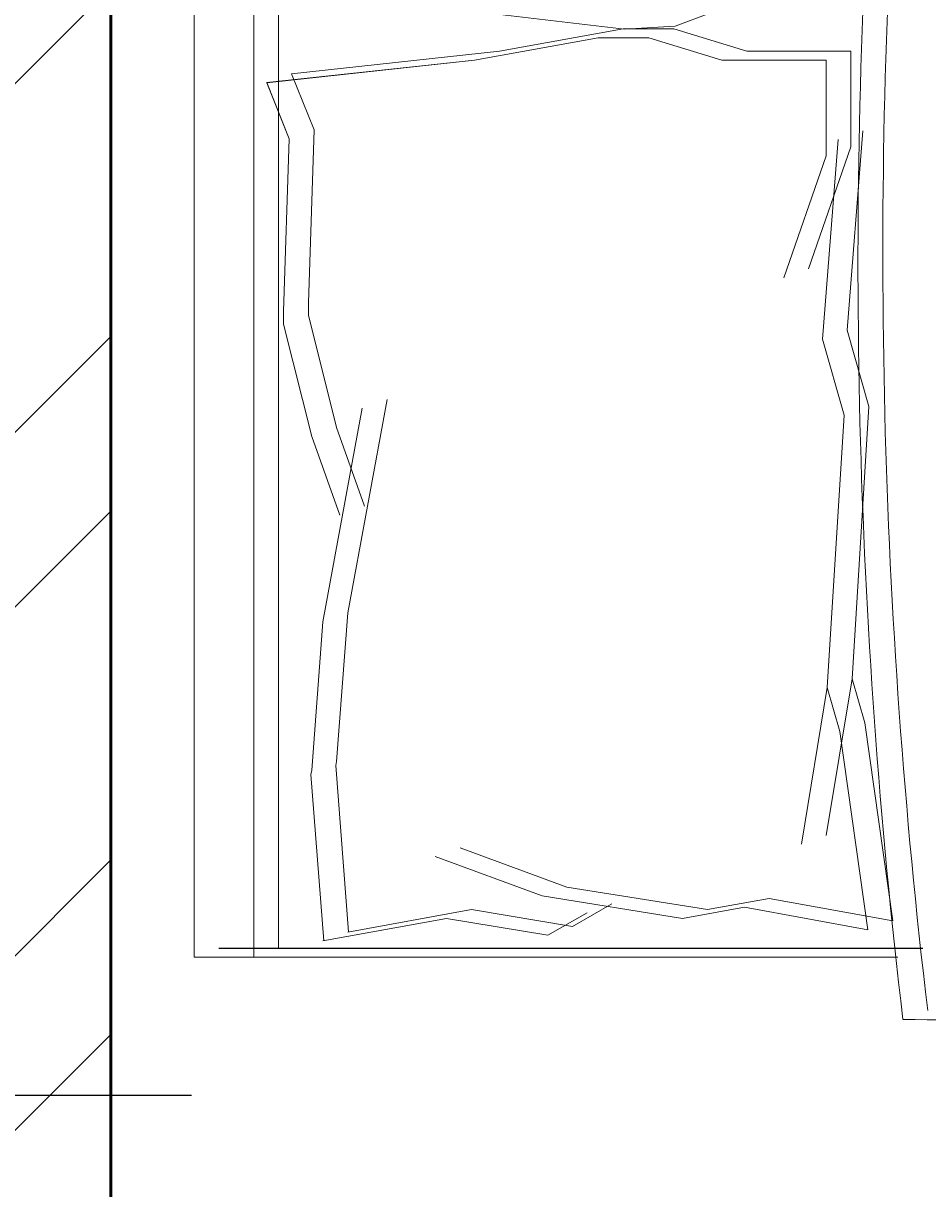
# Model space of a CAD drawing. Units: inches. Extents: x 963 to 2075, y 289 to 2657.
# Tile 37 of 98: x 1511 to 1534, y 1585 to 1615. Entities that reach past the tile are written whole.
import ezdxf

# ---------------------------------------------------------------- set-up
doc = ezdxf.new("R2010")
doc.units = ezdxf.units.IN
for name, color, linetype, lineweight in [('A-ANNO-DIMS', 2, 'Continuous', 18), ('A-FURN', 8, 'Continuous', 18), ('A-WALL', 7, 'Continuous', 50), ('A-WALL-PATT', 8, 'Continuous', 13)]:
    doc.layers.add(name, color=color, linetype=linetype, lineweight=lineweight)
doc.styles.get("Standard").update_dxf_attribs({"font": 'arial.ttf'})
doc.dimstyles.get("Standard").update_dxf_attribs({"dimtxt": 0.18, "dimasz": 0.18, "dimexe": 0.18, "dimexo": 0.0625, "dimgap": 0.09, "dimtad": 0, "dimtih": 1, "dimtoh": 1, "dimdec": 4, "dimzin": 0, "dimdsep": 46, "dimtxsty": 'Standard', "dimcen": 0.09, "dimadec": 0, "dimazin": 0, "dimtfac": 1, "dimtdec": 4, "dimtofl": 0, "dimtmove": 0, "dimatfit": 3, "dimfxl": 1, "dimtolj": 1, "dimtzin": 0, "dimarcsym": 0})

# ---------------------------------------------------------------- blocks, each defined once
blk = doc.blocks.new('BED-DOUBLE')
for p, q in [((1236.761, 2450.748), (1254.872, 2450.748)), ((1236.761, 2450.748), (1254.872, 2450.748)), ((1253.338, 2450.748), (1253.338, 2402.958)), ((1253.338, 2450.748), (1253.338, 2402.958)), ((1254.872, 2450.748), (1254.872, 2402.729)), ((1236.122, 2450.52), (1254.232, 2450.52)), ((1236.122, 2450.519), (1254.232, 2450.519)), ((1252.699, 2450.52), (1252.699, 2402.729)), ((1252.699, 2450.519), (1252.699, 2402.729)), ((1245.772, 2450.184), (1244.76, 2449.605)), ((1245.772, 2450.184), (1244.76, 2449.606)), ((1248.375, 2449.75), (1245.772, 2450.184)), ((1248.375, 2449.75), (1245.772, 2450.184)), ((1250.916, 2450.1), (1247.735, 2449.522)), ((1250.916, 2450.1), (1247.735, 2449.522)), ((1251.556, 2450.329), (1248.375, 2449.75)), ((1251.556, 2450.328), (1248.375, 2449.75)), ((1250.894, 2450.096), (1251.224, 2445.815)), ((1250.894, 2450.096), (1251.224, 2445.815)), ((1251.534, 2450.325), (1251.863, 2446.044)), ((1251.534, 2450.324), (1251.863, 2446.043)), ((1237.614, 2444.714), (1236.891, 2449.811)), ((1236.891, 2449.811), (1240.072, 2449.233)), ((1237.614, 2444.714), (1236.891, 2449.811)), ((1236.891, 2449.811), (1240.072, 2449.233)), ((1238.254, 2444.942), (1237.531, 2450.039)), ((1237.531, 2450.039), (1240.712, 2449.461)), ((1238.254, 2444.943), (1237.531, 2450.039)), ((1237.531, 2450.039), (1240.712, 2449.461)), ((1245.133, 2449.956), (1244.121, 2449.377)), ((1245.133, 2449.955), (1244.121, 2449.377)), ((1247.735, 2449.522), (1245.133, 2449.956)), ((1247.735, 2449.522), (1245.133, 2449.955)), ((1240.072, 2449.233), (1241.663, 2449.522)), ((1240.072, 2449.233), (1241.663, 2449.522)), ((1240.712, 2449.461), (1242.302, 2449.75)), ((1240.712, 2449.461), (1242.302, 2449.75)), ((1241.663, 2449.522), (1245.277, 2448.943)), ((1241.663, 2449.522), (1245.277, 2448.944)), ((1242.302, 2449.75), (1245.917, 2449.172)), ((1242.302, 2449.75), (1245.917, 2449.172)), ((1245.917, 2449.172), (1248.664, 2448.16)), ((1245.917, 2449.172), (1248.664, 2448.16)), ((1245.277, 2448.944), (1248.025, 2447.932)), ((1245.277, 2448.943), (1248.025, 2447.932)), ((1239.243, 2447.842), (1238.577, 2443.81)), ((1239.243, 2447.841), (1238.577, 2443.809)), ((1238.604, 2447.613), (1237.937, 2443.581)), ((1238.604, 2447.613), (1237.937, 2443.581)), ((1251.845, 2445.938), (1251.556, 2442.115)), ((1251.845, 2445.938), (1251.556, 2442.115)), ((1251.863, 2446.044), (1251.845, 2445.938)), ((1251.863, 2446.043), (1251.845, 2445.938)), ((1251.206, 2445.71), (1250.916, 2441.886)), ((1251.206, 2445.71), (1250.916, 2441.887)), ((1251.224, 2445.815), (1251.206, 2445.71)), ((1251.224, 2445.815), (1251.206, 2445.71)), ((1237.937, 2443.581), (1237.614, 2444.714)), ((1237.937, 2443.581), (1237.614, 2444.714)), ((1238.577, 2443.81), (1238.254, 2444.943)), ((1238.577, 2443.809), (1238.254, 2444.942)), ((1238.577, 2443.81), (1238.145, 2436.8)), ((1238.577, 2443.809), (1238.145, 2436.799)), ((1237.937, 2443.581), (1237.506, 2436.571)), ((1237.937, 2443.581), (1237.506, 2436.571)), ((1251.556, 2442.115), (1250.544, 2436.622)), ((1251.556, 2442.115), (1250.544, 2436.622)), ((1250.916, 2441.887), (1249.904, 2436.393)), ((1250.916, 2441.886), (1249.904, 2436.393)), ((1251.122, 2439.368), (1251.845, 2437.344)), ((1251.122, 2439.368), (1251.845, 2437.345)), ((1250.483, 2439.14), (1251.206, 2437.116)), ((1250.483, 2439.14), (1251.206, 2437.116)), ((1251.845, 2437.345), (1252.568, 2434.453)), ((1251.845, 2437.344), (1252.568, 2434.453)), ((1251.206, 2437.116), (1251.928, 2434.225)), ((1251.206, 2437.116), (1251.928, 2434.225)), ((1237.506, 2436.571), (1238.063, 2434.611)), ((1237.506, 2436.571), (1238.063, 2434.611)), ((1238.145, 2436.8), (1238.703, 2434.839)), ((1238.145, 2436.799), (1238.703, 2434.839)), ((1238.703, 2434.839), (1238.299, 2429.707)), ((1238.703, 2434.839), (1238.299, 2429.707)), ((1238.063, 2434.611), (1237.66, 2429.479)), ((1238.063, 2434.611), (1237.66, 2429.479)), ((1251.928, 2434.225), (1251.928, 2433.903)), ((1251.928, 2434.225), (1251.928, 2433.903)), ((1252.568, 2434.453), (1252.568, 2434.132)), ((1252.568, 2434.453), (1252.568, 2434.132)), ((1251.928, 2433.903), (1251.784, 2429.458)), ((1251.928, 2433.903), (1251.784, 2429.458)), ((1252.568, 2434.132), (1252.423, 2429.686)), ((1252.568, 2434.132), (1252.423, 2429.686)), ((1238.609, 2430.12), (1239.699, 2433.265)), ((1238.609, 2430.12), (1239.699, 2433.264)), ((1237.969, 2429.891), (1239.06, 2433.036)), ((1237.969, 2429.892), (1239.06, 2433.036)), ((1238.609, 2427.662), (1238.609, 2430.12)), ((1238.609, 2427.662), (1238.609, 2430.12)), ((1237.969, 2427.434), (1237.969, 2429.892)), ((1237.969, 2427.434), (1237.969, 2429.891)), ((1252.423, 2429.686), (1253.002, 2428.24)), ((1252.423, 2429.686), (1253.002, 2428.241)), ((1251.784, 2429.458), (1252.362, 2428.012)), ((1251.784, 2429.458), (1252.362, 2428.012)), ((1253.002, 2428.241), (1247.652, 2427.662)), ((1253.002, 2428.24), (1247.652, 2427.662)), ((1252.362, 2428.012), (1247.012, 2427.434)), ((1252.362, 2428.012), (1247.012, 2427.434)), ((1241.29, 2427.662), (1238.609, 2427.662)), ((1241.29, 2427.662), (1238.609, 2427.662)), ((1243.17, 2427.084), (1241.29, 2427.662)), ((1243.17, 2427.084), (1241.29, 2427.662)), ((1247.652, 2427.662), (1244.471, 2427.084)), ((1247.652, 2427.662), (1244.471, 2427.084)), ((1240.651, 2427.434), (1237.969, 2427.434)), ((1240.651, 2427.434), (1237.969, 2427.434)), ((1242.53, 2426.856), (1240.651, 2427.434)), ((1242.53, 2426.856), (1240.651, 2427.434)), ((1247.012, 2427.434), (1243.832, 2426.856)), ((1247.012, 2427.434), (1243.832, 2426.856)), ((1244.471, 2427.084), (1243.17, 2427.084)), ((1244.471, 2427.084), (1243.17, 2427.084)), ((1242.495, 2426.787), (1240.655, 2426.093)), ((1242.495, 2426.787), (1240.655, 2426.093)), ((1243.794, 2426.868), (1242.495, 2426.787)), ((1243.794, 2426.868), (1242.495, 2426.787)), ((1243.832, 2426.856), (1242.53, 2426.856)), ((1243.832, 2426.856), (1242.53, 2426.856)), ((1247.005, 2426.489), (1243.794, 2426.868)), ((1247.005, 2426.49), (1243.794, 2426.868))]:
    blk.add_line(p, q)
for centre, radius, start, end in [((1234.775, 2369.061), 83.306, 88.72178, 95.60397), ((1234.775, 2369.062), 83.306, 88.72178, 95.60397), ((1072.819, 2432.864), 164.969, 356.08655, 6.78213), ((1072.819, 2432.864), 164.969, 356.08655, 6.78213), ((1072.18, 2432.636), 164.969, 356.08655, 6.78213), ((1072.18, 2432.636), 164.969, 356.08655, 6.78213)]:
    blk.add_arc(centre, radius, start, end)
blk = doc.blocks.new('*D15')
at = {"layer": 'A-ANNO-DIMS', "color": 0, "lineweight": -2, "transparency": 16777216}
for p, q in [((1515.003, 1643.505), (1502.653, 1643.505)), ((1502.833, 1643.325), (1502.833, 1615.775)), ((1502.833, 1587.861), (1502.833, 1615.411)), ((1515.003, 1587.681), (1502.653, 1587.681))]:
    blk.add_line(p, q, dxfattribs=at)
at = {"layer": 'A-ANNO-DIMS', "color": 0, "transparency": 16777216}
for points in [[(1502.803, 1643.325), (1502.863, 1643.325), (1502.833, 1643.505)], [(1502.803, 1587.861), (1502.863, 1587.861), (1502.833, 1587.681)]]:
    blk.add_solid(points, dxfattribs=at)
at = {"layer": 'Defpoints', "color": 0, "transparency": 16777216}
for p in [(1515.065, 1643.505), (1502.833, 1587.681), (1515.065, 1587.681)]:
    blk.add_point(p, dxfattribs=at)
at = {"layer": 'A-ANNO-DIMS', "color": 0, "transparency": 16777216, "insert": (1502.833, 1615.593), "char_height": 0.18, "attachment_point": 5}
blk.add_mtext('\\A1;56 TYP.', dxfattribs=at)

msp = doc.modelspace()

# ---------------------------------------------------------------- hatches: boundary and pattern name
at = {"layer": 'A-WALL-PATT'}
h = msp.add_hatch(dxfattribs=at)
h.set_pattern_fill('ANSI32', color=256)
h.paths.add_polyline_path([(1473.609, 2163.068), (1473.609, 2165.318), (1376.422, 2165.318), (1376.422, 2227.983), (1371.922, 2227.983), (1371.922, 2214.818), (1368.405, 2214.818), (1368.405, 2210.318), (1371.922, 2210.318), (1371.922, 2160.818), (1395.922, 2160.818), (1395.922, 2090.318), (1217.345, 2090.318), (1217.345, 2085.818), (1395.922, 2085.818), (1458.922, 2085.818), (1458.922, 2108.318), (1454.422, 2108.318), (1454.422, 2090.318), (1400.422, 2090.318), (1400.422, 2160.818), (1473.609, 2160.818)])
h.paths.add_polyline_path([(1649.422, 2210.318), (1653.225, 2210.318), (1653.225, 2214.818), (1649.422, 2214.818), (1649.422, 2227.983), (1644.922, 2227.983), (1644.922, 2165.318), (1550.099, 2165.318), (1550.099, 2160.818), (1620.922, 2160.818), (1620.922, 2112.818), (1555.446, 2112.818), (1555.446, 2108.318), (1584.327, 2108.318), (1584.327, 2084.916), (1588.827, 2084.916), (1588.827, 2108.318), (1625.422, 2108.318), (1667.951, 2108.318), (1667.951, 2022.667), (1588.827, 2022.667), (1588.827, 2047.408), (1584.327, 2047.408), (1584.327, 1996.003), (1588.827, 1996.003), (1588.827, 2018.318), (1667.951, 2018.167), (1667.951, 1928.318), (1625.422, 1928.318), (1625.422, 1923.818), (1672.451, 1923.818), (1672.451, 1928.318), (1672.451, 1946.663), (1785.446, 1946.663), (1785.446, 1951.163), (1743.034, 1951.163), (1743.034, 2017.922), (1841.422, 2017.922), (1841.422, 2014.775), (1845.922, 2014.775), (1845.922, 2017.922), (1905.922, 2017.922), (1905.922, 1987.511), (1910.422, 1987.511), (1910.422, 2022.422), (1910.422, 2068.517), (1905.922, 2068.517), (1905.922, 2022.422), (1845.922, 2022.422), (1845.922, 2025.851), (1843.672, 2025.851), (1841.422, 2025.851), (1841.422, 2022.422), (1743.034, 2022.422), (1743.034, 2084.031), (1768.451, 2084.031), (1785.446, 2084.031), (1785.446, 2088.531), (1672.451, 2088.531), (1672.451, 2112.818), (1667.951, 2112.818), (1625.422, 2112.818), (1625.422, 2160.818), (1649.422, 2160.818)])
h.paths.add_polyline_path([(1672.451, 2084.031), (1738.534, 2084.031), (1738.534, 1951.163), (1672.451, 1951.163)], flags=16)
h.paths.add_polyline_path([(1672.451, 2084.031), (1738.534, 2084.031), (1705.492, 2017.597)], flags=0)
h.paths.add_polyline_path([(1262.766, 2085.818), (1258.266, 2085.818), (1258.266, 2023.278), (1184.422, 2023.278), (1184.422, 2018.778), (1258.266, 2018.778), (1258.266, 1950.818), (1262.766, 1950.818)])
h.paths.add_polyline_path([(1312.266, 2085.818), (1307.766, 2085.818), (1307.766, 1950.818), (1312.266, 1950.818)])
h.paths.add_polyline_path([(1458.922, 1950.818), (1395.922, 1950.818), (1216.568, 1950.818), (1216.568, 1946.318), (1346.422, 1946.318), (1395.922, 1946.318), (1395.922, 1875.818), (1371.922, 1875.818), (1371.922, 1826.318), (1368.931, 1826.318), (1368.931, 1821.818), (1371.922, 1821.818), (1371.922, 1813.622), (1376.422, 1813.622), (1376.422, 1871.318), (1474.504, 1871.318), (1474.504, 1873.568), (1474.504, 1875.818), (1400.422, 1875.818), (1400.422, 1946.318), (1454.422, 1946.318), (1454.422, 1928.318), (1458.922, 1928.318)])
h.paths.add_polyline_path([(1184.422, 2120.778), (1167.922, 2120.778), (1167.922, 2134.812), (1165.672, 2134.812), (1163.422, 2134.812), (1163.422, 2120.778), (1119.922, 2120.778), (1119.922, 2098.095), (1124.422, 2098.095), (1124.422, 2116.278), (1167.922, 2116.278), (1179.922, 2116.278), (1179.922, 2045.916), (1184.422, 2045.916), (1184.422, 2090.318), (1184.422, 2116.278)])
h.paths.add_polyline_path([(1124.422, 2018.778), (1179.922, 2018.778), (1179.922, 2016.294), (1184.422, 2016.294), (1184.422, 2023.278), (1184.422, 2026.588), (1182.172, 2026.588), (1179.922, 2026.588), (1179.922, 2023.278), (1124.422, 2023.278), (1124.422, 2074.095), (1119.922, 2074.095), (1119.922, 2018.778), (1119.922, 1979.633), (1124.422, 1979.633)])
h.paths.add_polyline_path([(1184.422, 1925.778), (1184.422, 1946.318), (1184.422, 1996.073), (1182.172, 1996.073), (1179.922, 1996.073), (1179.922, 1925.778), (1124.422, 1925.778), (1124.422, 1955.633), (1119.922, 1955.502), (1119.922, 1921.278), (1158.922, 1921.278), (1158.922, 1909.983), (1163.422, 1909.983), (1163.422, 1921.278), (1184.422, 1921.278)])
h.paths.add_polyline_path([(1341.449, 1826.318), (1163.422, 1826.318), (1163.422, 1849.983), (1158.922, 1849.983), (1158.922, 1821.818), (1158.922, 1804.033), (1163.422, 1804.033), (1163.422, 1821.818), (1341.449, 1821.818)])
h.paths.add_polyline_path([(1222.981, 1713.818), (1163.422, 1713.818), (1163.422, 1744.033), (1161.172, 1744.033), (1158.922, 1744.033), (1158.922, 1713.818), (1119.922, 1713.818), (1119.922, 1694.65), (1124.422, 1694.65), (1124.422, 1709.318), (1158.922, 1709.318), (1222.981, 1709.318)])
h.paths.add_polyline_path([(1328.422, 1713.818), (1252.042, 1713.818), (1252.042, 1711.568), (1252.042, 1709.318), (1256.422, 1709.318), (1256.422, 1547.318), (1232.937, 1547.318), (1232.937, 1545.068), (1232.937, 1542.818), (1292.422, 1542.818), (1292.422, 1527.634), (1296.922, 1527.634), (1296.922, 1542.818), (1299.464, 1542.818), (1299.464, 1547.318), (1260.922, 1547.318), (1260.922, 1658.318), (1343.661, 1658.318), (1343.661, 1660.568), (1343.661, 1662.818), (1328.422, 1662.818), (1328.422, 1676.589), (1327.402, 1676.589), (1323.922, 1676.589), (1323.922, 1662.818), (1260.922, 1662.818), (1260.922, 1709.318), (1323.922, 1709.318), (1323.922, 1699.851), (1328.422, 1699.851)])
h.paths.add_polyline_path([(1649.422, 1875.818), (1625.422, 1875.818), (1625.422, 1928.318), (1620.922, 1928.318), (1588.827, 1928.318), (1588.827, 1950.59), (1584.327, 1950.59), (1584.327, 1928.318), (1555.446, 1928.318), (1555.446, 1923.818), (1620.922, 1923.818), (1620.922, 1875.818), (1548.952, 1875.818), (1548.952, 1873.568), (1548.952, 1871.318), (1644.922, 1871.318), (1644.922, 1813.622), (1649.422, 1813.622), (1649.422, 1821.818), (1652.045, 1821.818), (1652.045, 1824.068), (1652.045, 1826.318), (1649.422, 1826.318)])
h.paths.add_polyline_path([(1512.922, 1871.318), (1516.476, 1871.318), (1516.476, 1875.818), (1512.922, 1875.818), (1512.922, 1923.818), (1512.922, 1928.318), (1512.922, 1930.827), (1508.422, 1930.827), (1508.422, 1875.818), (1504.411, 1875.818), (1504.411, 1871.318), (1508.422, 1871.318), (1508.422, 1713.818), (1376.422, 1713.818), (1376.422, 1743.325), (1371.922, 1743.325), (1371.922, 1709.318), (1371.922, 1706.01), (1376.422, 1706.01), (1376.422, 1709.318), (1508.422, 1709.318), (1508.422, 1547.318), (1501.871, 1547.318), (1501.871, 1542.818), (1508.422, 1542.818), (1508.422, 1482.818), (1508.422, 1436.318), (1512.922, 1436.318), (1512.922, 1542.818), (1519.318, 1542.818), (1519.318, 1545.068), (1519.318, 1547.318), (1512.922, 1547.318), (1512.922, 1709.318), (1644.922, 1709.318), (1644.922, 1707.548), (1649.422, 1707.548), (1649.422, 1709.318), (1649.422, 1743.325), (1644.922, 1743.325), (1644.922, 1713.818), (1512.922, 1713.818)])
h.paths.add_polyline_path([(1129.884, 1545.068), (1129.884, 1547.318), (1124.422, 1547.318), (1095.922, 1547.318), (1095.922, 1614.818), (1124.422, 1614.818), (1124.422, 1619.318), (1095.922, 1619.318), (1091.422, 1619.318), (1091.422, 1542.818), (1095.922, 1542.818), (1119.922, 1542.818), (1129.884, 1542.818)])
h.paths.add_polyline_path([(1208.422, 1542.818), (1211.74, 1542.818), (1211.74, 1547.318), (1198.851, 1547.318), (1198.851, 1542.818), (1203.922, 1542.818), (1203.922, 1478.318), (1208.422, 1478.318), (1296.922, 1478.318), (1296.922, 1503.634), (1292.422, 1503.634), (1292.422, 1482.818), (1208.422, 1482.818)])
h.paths.add_polyline_path([(1430.422, 1542.818), (1435.699, 1542.818), (1435.699, 1545.068), (1435.699, 1547.318), (1422.658, 1547.318), (1422.658, 1545.068), (1422.658, 1542.818), (1425.922, 1542.818), (1425.922, 1482.857), (1341.922, 1482.857), (1341.922, 1502.732), (1337.422, 1502.732), (1337.422, 1478.357), (1425.922, 1478.357), (1425.922, 1440.818), (1425.922, 1436.318), (1430.422, 1436.318)])
h.paths.add_polyline_path([(1698.482, 2004.259), (1727.695, 2004.259), (1727.695, 2022.916), (1698.482, 2022.916)], flags=8)

# ---------------------------------------------------------------- linework, layer by layer
at = {"layer": 'A-WALL'}
msp.add_line((1512.922, 1547.318), (1512.922, 1709.318), dxfattribs=at)

# ---------------------------------------------------------------- block references
at = {"layer": 'A-FURN', "rotation": 180}
msp.add_blockref('BED-DOUBLE', (2769.937, 4041.99), dxfattribs=at)

# ---------------------------------------------------------------- dimensions: what is measured, and where the dimension line sits
at = {"layer": 'A-ANNO-DIMS'}
dim = msp.add_linear_dim(base=(1502.833, 1587.681), p1=(1515.065, 1643.505), p2=(1515.065, 1587.681), angle=270, text='<> TYP.', dimstyle='Standard', override={"dimdec": 0, "dimlfac": 1, "dimrnd": 0, "dimzin": 0, "dimdsep": 46, "dimlunit": 2}, dxfattribs=at)
dim.commit()
dim.dimension.update_dxf_attribs({"geometry": '*D15', "text_midpoint": (1502.833, 1615.593)})

doc.saveas('drawing.dxf')
